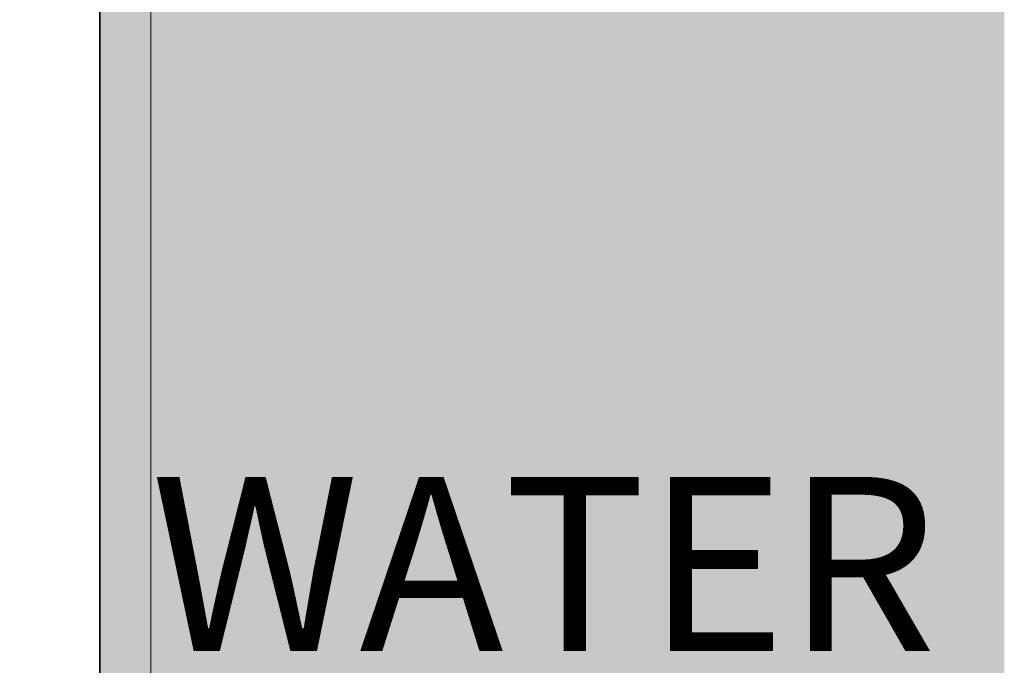
# Model space of a CAD drawing. Units: inches. Extents: x 1704 to 6393, y -157 to 1172.
# Tile 52 of 122: x 1892 to 1969, y 819 to 870. Entities that reach past the tile are written whole.
import ezdxf

# ---------------------------------------------------------------- set-up
doc = ezdxf.new("R2010")
doc.units = ezdxf.units.IN
doc.header["$MEASUREMENT"] = 0
for name, color, linetype, lineweight in [('A-ANNO-DIMS', 7, 'Continuous', 13), ('A-AREA-IDEN', 7, 'Continuous', 18), ('C-PROP', 7, 'Continuous', 35), ('L-HRDS', 8, 'Continuous', 18)]:
    doc.layers.add(name, color=color, linetype=linetype, lineweight=lineweight)
doc.layers.add('L-HRDS-PATT', color=9, linetype='Continuous', lineweight=13, true_color=0xc5c1ba)
doc.layers.add('L-WATR-PATT', color=143, linetype='Continuous', lineweight=13, true_color=0x7ab0df)
doc.styles.get("Standard").update_dxf_attribs({"font": 'arial.ttf'})
doc.dimstyles.get("Standard").update_dxf_attribs({"dimtxt": 6, "dimasz": 2, "dimexe": 0.18, "dimexo": 0.0625, "dimgap": 0.09, "dimtad": 0, "dimtih": 1, "dimtoh": 1, "dimdec": 1, "dimzin": 0, "dimdsep": 46, "dimlunit": 3, "dimtxsty": 'Standard', "dimblk": 'ARCHTICK', "dimcen": 0.09, "dimadec": 0, "dimazin": 0, "dimtfac": 1, "dimtdec": 1, "dimtofl": 0, "dimtmove": 0, "dimatfit": 3, "dimfxl": 1, "dimtolj": 1, "dimtzin": 0, "dimarcsym": 0})

# ---------------------------------------------------------------- blocks, each defined once
blk = doc.blocks.new('_ArchTick')
at = {"color": 0, "linetype": 'ByBlock', "const_width": 0.15}
blk.add_lwpolyline([(-0.5, -0.5), (0.5, 0.5)], dxfattribs=at)
blk = doc.blocks.new('*D93')
at = {"layer": 'A-ANNO-DIMS', "color": 0, "lineweight": -2, "transparency": 16777216}
for p, q in [((2605.286, 895.213), (1829.698, 895.213)), ((1829.878, 895.213), (1829.878, 495.866)), ((1829.878, 90.213), (1829.878, 489.56)), ((2605.286, 90.213), (1829.698, 90.213))]:
    blk.add_line(p, q, dxfattribs=at)
at = {"layer": 'Defpoints', "color": 0, "lineweight": -3, "transparency": 16777216}
for p in [(2605.349, 895.213), (1829.878, 90.213), (2605.349, 90.213)]:
    blk.add_point(p, dxfattribs=at)
at = {"layer": 'A-ANNO-DIMS', "color": 0, "lineweight": -2, "transparency": 16777216, "xscale": 2, "yscale": 2, "zscale": 2}
for p, rotation in [((1829.878, 895.213), 90), ((1829.878, 90.213), 270)]:
    blk.add_blockref('_ArchTick', p, dxfattribs=dict(at, rotation=rotation))
at = {"layer": 'A-ANNO-DIMS', "color": 0, "transparency": 16777216, "insert": (1829.878, 492.713), "char_height": 6, "attachment_point": 5}
blk.add_mtext('\\A1;805', dxfattribs=at)

msp = doc.modelspace()

# ---------------------------------------------------------------- hatches: boundary and pattern name
at = {"layer": 'L-HRDS-PATT'}
h = msp.add_hatch(color=256, dxfattribs=at)
h.dxf.hatch_style = 1
h.paths.add_polyline_path([(1902.349, 887.213), (1898.349, 887.213), (1898.349, 719.213), (1902.349, 719.213)])
at = {"layer": 'L-WATR-PATT'}
h = msp.add_hatch(color=256, dxfattribs=at)
h.dxf.hatch_style = 1
h.paths.add_polyline_path([(1969.349, 887.213), (1902.349, 887.213), (1902.349, 719.213), (1969.349, 719.213)])

# ---------------------------------------------------------------- linework, layer by layer
at = {"layer": 'C-PROP'}
msp.add_line((1898.349, -3.787), (1898.349, 1033.213), dxfattribs=at)
at = {"layer": 'L-HRDS'}
msp.add_line((1902.349, 887.213), (1902.349, 719.213), dxfattribs=at)

# ---------------------------------------------------------------- texts
at = {"layer": 'A-AREA-IDEN'}
msp.add_text('WATER', height=13.6672, dxfattribs=at).set_placement((1902.349, 820.194))
msp.add_text('WATER', height=13.6672, dxfattribs=at).set_placement((1902.349, 820.194))

# ---------------------------------------------------------------- dimensions: what is measured, and where the dimension line sits
at = {"layer": 'A-ANNO-DIMS'}
dim = msp.add_linear_dim(base=(1829.878, 90.213), p1=(2605.349, 895.213), p2=(2605.349, 90.213), angle=90, dimstyle='Standard', override={"dimdec": 0, "dimlfac": 1, "dimrnd": 0, "dimzin": 0, "dimdsep": 46, "dimlunit": 2}, dxfattribs=at)
dim.commit()
dim.dimension.update_dxf_attribs({"geometry": '*D93', "text_midpoint": (1829.878, 492.713)})

doc.saveas('drawing.dxf')
